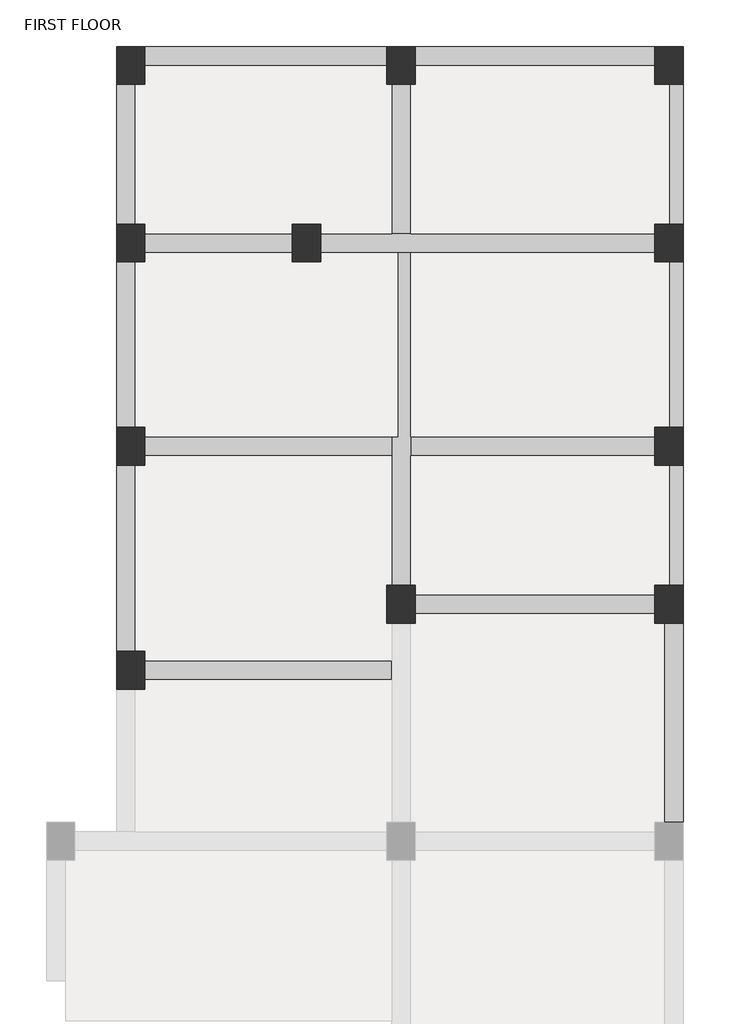
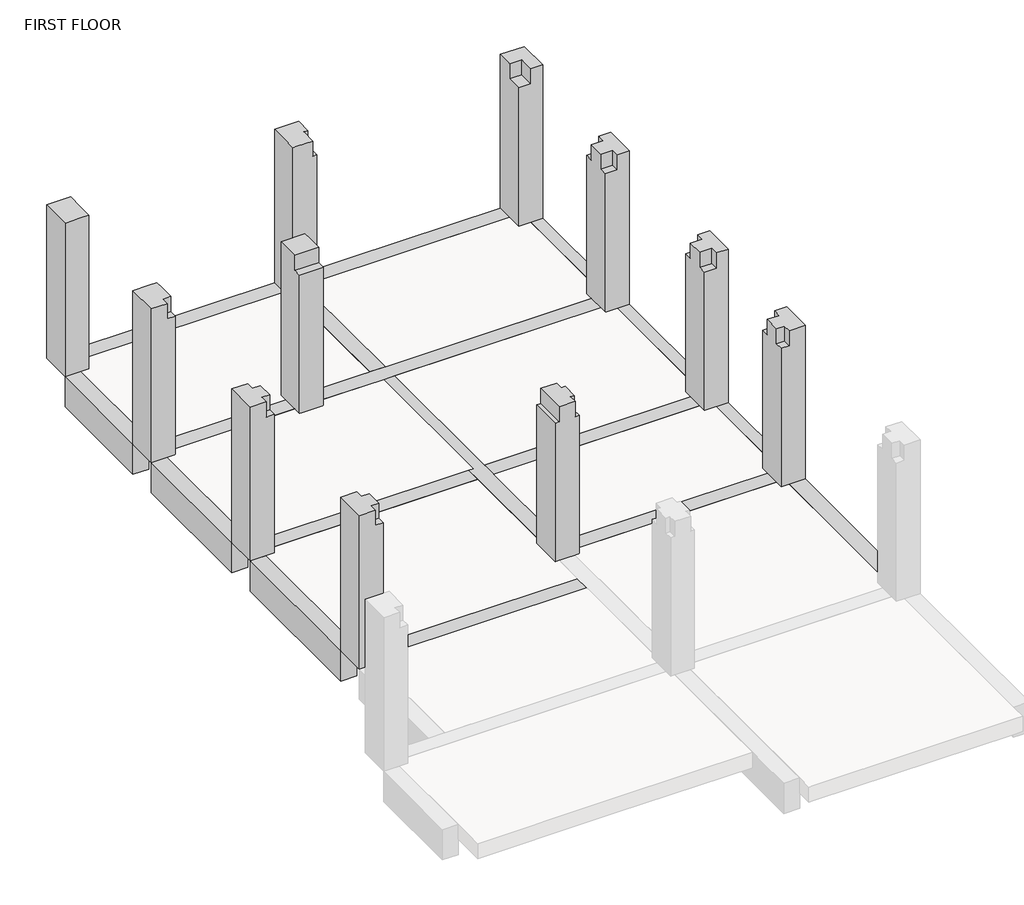
# One storey, part 2 of 2: 17 beams, 11 columns.
"""IFC4 building model written with IfcOpenShell, lengths in millimetres."""

from ifc_helpers import new_model, si_unit, frame, origin, place, context, project, spatial, polyline, outline, extrude, faceted_brep, element, save

model = new_model("IFC4")

# Units and contexts
model_context = context("Model", 3, world=origin())
ifc_project = project(units=[si_unit("LENGTHUNIT", "METRE", prefix="MILLI")], contexts=[model_context])

# Site, building, storey
site = spatial("IfcSite", under=ifc_project)
building = spatial("IfcBuilding", under=site)
storey = spatial("IfcBuildingStorey", under=building, Name="FIRST FLOOR", Elevation=3000.0)

# Beams
placement = place(None, origin())
element("IfcBeam", 1, ObjectType="M_Concrete-Rectangular Beam : 300 x 600mm", at=placement, inside=storey, context=model_context, shape_type="Brep", body=[
    faceted_brep([(-2096.635935, 10150.0657956, 3000.0), (-2096.635935, 10450.0657956, 3000.0), (-5925.9642664, 10450.0657956, 3000.0), (-5925.9642664, 10150.0657956, 3000.0), (-2096.635935, 10150.0657956, 2400.0), (-2096.635935, 10150.0657956, 2700.0), (-5925.9642664, 10150.0657956, 2700.0), (-5925.9642664, 10150.0657956, 2400.0), (-2096.635935, 10450.0657956, 2400.0), (-5925.9642664, 10450.0657956, 2400.0)], [[[0, 1, 2, 3]], [[4, 5, 0, 3, 6, 7]], [[8, 4, 7, 9]], [[1, 8, 9, 2]], [[2, 9, 7, 6, 3]], [[1, 0, 5, 4, 8]]]),
])
element("IfcBeam", 2, ObjectType="M_Concrete-Rectangular Beam : 300 x 600mm", at=placement, inside=storey, context=model_context, shape_type="SweptSolid", body=[
    extrude(outline(polyline([(2143.5134108, 10450.0657956), (2143.5134108, 10150.0657956), (-1646.635935, 10150.0657956), (-1646.635935, 10450.0657956), (2143.5134108, 10450.0657956)])), frame((0.0, 0.0, 2400.0), z_axis=(0.0, 0.0, 1.0), x_axis=(1.0, 0.0, 0.0)), (0.0, 0.0, 1.0), 600.0),
])
element("IfcBeam", 3, ObjectType="M_Concrete-Rectangular Beam : 300 x 600mm", at=placement, inside=storey, context=model_context, shape_type="Brep", body=[
    faceted_brep([(-6375.9642664, 7641.506653, 3000.0), (-6075.9642664, 7641.506653, 3000.0), (-6075.9642664, 9850.0657956, 3000.0), (-6375.9642664, 9850.0657956, 3000.0), (-6375.9642664, 7641.506653, 2400.0), (-6375.9642664, 9850.0657956, 2400.0), (-6075.9642664, 7641.506653, 2400.0), (-6075.9642664, 9850.0657956, 2400.0), (-6075.9642664, 7641.506653, 2700.0), (-6075.9642664, 9850.0657956, 2700.0)], [[[0, 1, 2, 3]], [[4, 0, 3, 5]], [[6, 4, 5, 7]], [[1, 8, 6, 7, 9, 2]], [[2, 9, 7, 5, 3]], [[1, 0, 4, 6, 8]]]),
])
element("IfcBeam", 4, ObjectType="M_Concrete-Rectangular Beam : 300 x 600mm", at=placement, inside=storey, context=model_context, shape_type="SweptSolid", body=[
    extrude(outline(polyline([(-6075.9642664, 4424.5351605), (-6375.9642664, 4424.5351605), (-6375.9642664, 7041.506653), (-6075.9642664, 7041.506653), (-6075.9642664, 4424.5351605)])), frame((0.0, 0.0, 2400.0), z_axis=(0.0, 0.0, 1.0), x_axis=(1.0, 0.0, 0.0)), (0.0, 0.0, 1.0), 600.0),
])
element("IfcBeam", 5, ObjectType="M_Concrete-Rectangular Beam : 300 x 600mm", at=placement, inside=storey, context=model_context, shape_type="SweptSolid", body=[
    extrude(outline(polyline([(-6075.9642664, 881.5941646), (-6375.9642664, 881.5941646), (-6375.9642664, 3824.5351605), (-6075.9642664, 3824.5351605), (-6075.9642664, 881.5941646)])), frame((0.0, 0.0, 2400.0), z_axis=(0.0, 0.0, 1.0), x_axis=(1.0, 0.0, 0.0)), (0.0, 0.0, 1.0), 600.0),
])
element("IfcBeam", 6, ObjectType="M_Concrete-Rectangular Beam : 300 x 600mm", at=placement, inside=storey, context=model_context, shape_type="SweptSolid", body=[
    extrude(outline(polyline([(2293.5134108, 1328.1057379), (2593.5134108, 1328.1057379), (2593.5134108, -1823.3693625), (2293.5134108, -1823.3693625), (2293.5134108, 1328.1057379)])), frame((0.0, 0.0, 2400.0), z_axis=(0.0, 0.0, 1.0), x_axis=(1.0, 0.0, 0.0)), (0.0, 0.0, 1.0), 600.0),
])
element("IfcBeam", 7, ObjectType="M_Concrete-Rectangular Beam : 300 x 600mm", at=placement, inside=storey, context=model_context, shape_type="SweptSolid", body=[
    extrude(outline(polyline([(2400.0, 2293.5134108), (2400.0, 2593.5134108), (3000.0, 2593.5134108), (3000.0, 2368.5134108), (2700.0, 2368.5134108), (2700.0, 2293.5134108), (2400.0, 2293.5134108)])), frame((0.0, 1928.1057379, 0.0), z_axis=(0.0, 1.0, 0.0), x_axis=(0.0, 0.0, 1.0)), (0.0, 0.0, 1.0), 1896.4294226),
])
element("IfcBeam", 8, ObjectType="M_Concrete-Rectangular Beam : 300 x 600mm", at=placement, inside=storey, context=model_context, shape_type="SweptSolid", body=[
    extrude(outline(polyline([(2400.0, 2293.5134108), (2400.0, 2593.5134108), (3000.0, 2593.5134108), (3000.0, 2368.5134108), (2700.0, 2368.5134108), (2700.0, 2293.5134108), (2400.0, 2293.5134108)])), frame((0.0, 4424.5351605, 0.0), z_axis=(0.0, 1.0, 0.0), x_axis=(0.0, 0.0, 1.0)), (0.0, 0.0, 1.0), 2616.9714925),
])
element("IfcBeam", 9, ObjectType="M_Concrete-Rectangular Beam : 300 x 600mm", at=placement, inside=storey, context=model_context, shape_type="SweptSolid", body=[
    extrude(outline(polyline([(2400.0, 2293.5134108), (2400.0, 2593.5134108), (3000.0, 2593.5134108), (3000.0, 2368.5134108), (2700.0, 2368.5134108), (2700.0, 2293.5134108), (2400.0, 2293.5134108)])), frame((0.0, 7641.506653, 0.0), z_axis=(0.0, 1.0, 0.0), x_axis=(0.0, 0.0, 1.0)), (0.0, 0.0, 1.0), 2208.5591426),
])
element("IfcBeam", 10, ObjectType="M_Concrete-Rectangular Beam : 300 x 600mm", at=placement, inside=storey, context=model_context, shape_type="Brep", body=[
    faceted_brep([(-3596.635935, 7191.506653, 3000.0), (-3596.635935, 7491.506653, 3000.0), (-5925.9642664, 7491.506653, 3000.0), (-5925.9642664, 7191.506653, 3000.0), (-3596.635935, 7191.506653, 2400.0), (-5925.9642664, 7191.506653, 2400.0), (-3596.635935, 7491.506653, 2400.0), (-5925.9642664, 7491.506653, 2400.0), (-3596.635935, 7491.506653, 2700.0), (-5925.9642664, 7491.506653, 2700.0)], [[[0, 1, 2, 3]], [[4, 0, 3, 5]], [[6, 4, 5, 7]], [[1, 8, 6, 7, 9, 2]], [[2, 9, 7, 5, 3]], [[1, 0, 4, 6, 8]]]),
])
element("IfcBeam", 11, ObjectType="M_Concrete-Rectangular Beam : 300 x 600mm", at=placement, inside=storey, context=model_context, shape_type="Brep", body=[
    faceted_brep([(-3146.635935, 7491.506653, 3000.0), (-3146.635935, 7191.506653, 3000.0), (-1928.7254278, 7191.506653, 3000.0), (-1721.635935, 7191.506653, 3000.0), (2143.5134108, 7191.506653, 3000.0), (2143.5134108, 7491.506653, 3000.0), (-1721.635935, 7491.506653, 3000.0), (-2021.635935, 7491.506653, 3000.0), (-3146.635935, 7491.506653, 2400.0), (-3146.635935, 7491.506653, 2700.0), (2143.5134108, 7491.506653, 2400.0), (-1721.635935, 7491.506653, 2400.0), (-2021.635935, 7491.506653, 2400.0), (-3146.635935, 7191.506653, 2400.0), (2143.5134108, 7191.506653, 2400.0), (-1721.635935, 7191.506653, 2400.0), (-2021.635935, 7191.506653, 2400.0)], [[[0, 1, 2, 3, 4, 5, 6, 7]], [[8, 9, 0, 7, 6, 5, 10, 11, 12]], [[13, 8, 12, 11, 10, 14, 15, 16]], [[1, 13, 16, 15, 14, 4, 3, 2]], [[1, 0, 9, 8, 13]], [[4, 14, 10, 5]]]),
])
element("IfcBeam", 12, ObjectType="M_Concrete-Rectangular Beam : 300 x 600mm", at=placement, inside=storey, context=model_context, shape_type="SweptSolid", body=[
    extrude(outline(polyline([(-1646.635935, 1478.1057379), (-1646.635935, 1778.1057379), (2143.5134108, 1778.1057379), (2143.5134108, 1478.1057379), (-1646.635935, 1478.1057379)])), frame((0.0, 0.0, 2400.0), z_axis=(0.0, 0.0, 1.0), x_axis=(1.0, 0.0, 0.0)), (0.0, 0.0, 1.0), 600.0),
])
element("IfcBeam", 13, ObjectType="M_Concrete-Rectangular Beam : 300 x 600mm", at=placement, inside=storey, context=model_context, shape_type="Brep", body=[
    faceted_brep([(-1721.635935, 9850.0657956, 3000.0), (-2021.635935, 9850.0657956, 3000.0), (-2021.635935, 7491.506653, 3000.0), (-1721.635935, 7491.506653, 3000.0), (-2021.635935, 9850.0657956, 2700.0), (-2021.635935, 9850.0657956, 2400.0), (-2021.635935, 7491.506653, 2400.0), (-2021.635935, 7491.506653, 2700.0), (-1721.635935, 9850.0657956, 2400.0), (-1721.635935, 7491.506653, 2400.0), (-1721.635935, 7491.506653, 2700.0)], [[[0, 1, 2, 3]], [[1, 4, 5, 6, 7, 2]], [[5, 8, 9, 6]], [[8, 0, 3, 10, 9]], [[0, 8, 5, 4, 1]], [[3, 2, 7, 6, 9, 10]]]),
])
element("IfcBeam", 14, ObjectType="M_Concrete-Rectangular Beam : 300 x 600mm", at=placement, inside=storey, context=model_context, shape_type="Brep", body=[
    faceted_brep([(-2021.635935, 1928.1057379, 3000.0), (-1721.635935, 1928.1057379, 3000.0), (-1721.635935, 3974.5351605, 3000.0), (-1721.635935, 4274.5351605, 3000.0), (-1721.635935, 7191.506653, 3000.0), (-1928.7254278, 7191.506653, 3000.0), (-1928.7254278, 4274.5351605, 3000.0), (-2021.635935, 4274.5351605, 3000.0), (-2021.635935, 3974.5351605, 3000.0), (-1721.635935, 1928.1057379, 2400.0), (-1721.635935, 3974.5351605, 2400.0), (-1721.635935, 4274.5351605, 2400.0), (-1721.635935, 7191.506653, 2400.0), (-1721.635935, 7191.506653, 2700.0), (-2021.635935, 1928.1057379, 2400.0), (-2021.635935, 3974.5351605, 2400.0), (-2021.635935, 4274.5351605, 2400.0), (-2021.635935, 7191.506653, 2400.0), (-2021.635935, 4274.5351605, 2700.0), (-2021.635935, 7191.506653, 2700.0), (-1928.7254278, 7191.506653, 2700.0), (-1928.7254278, 4274.5351605, 2700.0)], [[[0, 1, 2, 3, 4, 5, 6, 7, 8]], [[1, 9, 10, 11, 12, 13, 4, 3, 2]], [[9, 14, 15, 16, 17, 12, 11, 10]], [[14, 0, 8, 7, 18, 19, 17, 16, 15]], [[0, 14, 9, 1]], [[4, 13, 12, 17, 19, 20, 5]], [[21, 20, 19, 18]], [[20, 21, 6, 5]], [[6, 21, 18, 7]]]),
])
element("IfcBeam", 15, ObjectType="M_Concrete-Rectangular Beam : 300 x 600mm", at=placement, inside=storey, context=model_context, shape_type="Brep", body=[
    faceted_brep([(-5925.9642664, 731.5941646, 3000.0), (-5925.9642664, 431.5941646, 3000.0), (-2021.635935, 431.5941646, 3000.0), (-2021.635935, 731.5941646, 3000.0), (-5925.9642664, 431.5941646, 2400.0), (-2021.635935, 431.5941646, 2400.0), (-2021.635935, 431.5941646, 2700.0), (-5925.9642664, 731.5941646, 2400.0), (-2021.635935, 731.5941646, 2400.0), (-2021.635935, 731.5941646, 2700.0)], [[[0, 1, 2, 3]], [[1, 4, 5, 6, 2]], [[4, 7, 8, 5]], [[7, 0, 3, 9, 8]], [[0, 7, 4, 1]], [[3, 2, 6, 5, 8, 9]]]),
])
element("IfcBeam", 16, ObjectType="M_Concrete-Rectangular Beam : 300 x 600mm", at=placement, inside=storey, context=model_context, shape_type="Brep", body=[
    faceted_brep([(-5925.9642664, 4274.5351605, 3000.0), (-5925.9642664, 3974.5351605, 3000.0), (-2021.635935, 3974.5351605, 3000.0), (-2021.635935, 4274.5351605, 3000.0), (-5925.9642664, 3974.5351605, 2400.0), (-2021.635935, 3974.5351605, 2400.0), (-2021.635935, 3974.5351605, 2700.0), (-5925.9642664, 4274.5351605, 2400.0), (-2021.635935, 4274.5351605, 2400.0), (-2021.635935, 4274.5351605, 2700.0)], [[[0, 1, 2, 3]], [[1, 4, 5, 6, 2]], [[4, 7, 8, 5]], [[7, 0, 3, 9, 8]], [[0, 7, 4, 1]], [[3, 2, 6, 5, 8, 9]]]),
])
element("IfcBeam", 17, ObjectType="M_Concrete-Rectangular Beam : 300 x 600mm", at=placement, inside=storey, context=model_context, shape_type="Brep", body=[
    faceted_brep([(2143.5134108, 3974.5351605, 3000.0), (2143.5134108, 4274.5351605, 3000.0), (-1721.635935, 4274.5351605, 3000.0), (-1721.635935, 3974.5351605, 3000.0), (2143.5134108, 4274.5351605, 2400.0), (-1721.635935, 4274.5351605, 2400.0), (-1721.635935, 4274.5351605, 2700.0), (2143.5134108, 3974.5351605, 2400.0), (-1721.635935, 3974.5351605, 2400.0), (-1721.635935, 3974.5351605, 2700.0)], [[[0, 1, 2, 3]], [[1, 4, 5, 6, 2]], [[4, 7, 8, 5]], [[7, 0, 3, 9, 8]], [[0, 7, 4, 1]], [[3, 2, 6, 5, 8, 9]]]),
])

# Columns
element("IfcColumn", 18, ObjectType="M_Concrete-Rectangular-Column : 450 x 600mm", at=placement, inside=storey, context=model_context, shape_type="Brep", body=[
    faceted_brep([(-5925.9642664, 10450.0657956, 3000.0), (-5925.9642664, 9850.0657956, 3000.0), (-6375.9642664, 9850.0657956, 3000.0), (-6375.9642664, 10450.0657956, 3000.0), (-5925.9642664, 10450.0657956, 6048.0), (-5925.9642664, 10150.0657956, 6048.0), (-5925.9642664, 9850.0657956, 6048.0), (-5925.9642664, 9850.0657956, 5748.0), (-6075.9642664, 9850.0657956, 6048.0), (-6375.9642664, 9850.0657956, 6048.0), (-6375.9642664, 10450.0657956, 6048.0)], [[[0, 1, 2, 3]], [[1, 0, 4, 5, 6, 7]], [[2, 1, 7, 6, 8, 9]], [[3, 2, 9, 10]], [[0, 3, 10, 4]], [[10, 9, 8, 6, 5, 4]]]),
])
element("IfcColumn", 19, ObjectType="M_Concrete-Rectangular-Column : 450 x 600mm", at=placement, inside=storey, context=model_context, shape_type="Brep", body=[
    faceted_brep([(-5925.9642664, 7641.506653, 3000.0), (-5925.9642664, 7041.506653, 3000.0), (-6375.9642664, 7041.506653, 3000.0), (-6375.9642664, 7641.506653, 3000.0), (-5925.9642664, 7641.506653, 5748.0), (-5925.9642664, 7641.506653, 6048.0), (-5925.9642664, 7491.506653, 6048.0), (-5925.9642664, 7191.506653, 6048.0), (-5925.9642664, 7191.506653, 5748.0), (-5925.9642664, 7041.506653, 5748.0), (-6075.9642664, 7041.506653, 5748.0), (-6075.9642664, 7041.506653, 6048.0), (-6375.9642664, 7041.506653, 6048.0), (-6375.9642664, 7641.506653, 6048.0), (-6075.9642664, 7641.506653, 6048.0), (-6075.9642664, 7191.506653, 6048.0), (-6075.9642664, 7191.506653, 5748.0)], [[[0, 1, 2, 3]], [[1, 0, 4, 5, 6, 7, 8, 9]], [[2, 1, 9, 10, 11, 12]], [[3, 2, 12, 13]], [[0, 3, 13, 14, 5, 4]], [[13, 12, 11, 15, 7, 6, 5, 14]], [[16, 10, 9, 8]], [[15, 16, 8, 7]], [[16, 15, 11, 10]]]),
])
element("IfcColumn", 20, ObjectType="M_Concrete-Rectangular-Column : 450 x 600mm", at=placement, inside=storey, context=model_context, shape_type="Brep", body=[
    faceted_brep([(-5925.9642664, 4424.5351605, 3000.0), (-5925.9642664, 3824.5351605, 3000.0), (-6375.9642664, 3824.5351605, 3000.0), (-6375.9642664, 4424.5351605, 3000.0), (-5925.9642664, 4424.5351605, 5748.0), (-5925.9642664, 4274.5351605, 5748.0), (-5925.9642664, 4274.5351605, 6048.0), (-5925.9642664, 3974.5351605, 6048.0), (-5925.9642664, 3974.5351605, 5748.0), (-5925.9642664, 3824.5351605, 5748.0), (-6075.9642664, 3824.5351605, 5748.0), (-6075.9642664, 3824.5351605, 6048.0), (-6375.9642664, 3824.5351605, 6048.0), (-6375.9642664, 4424.5351605, 6048.0), (-6075.9642664, 4424.5351605, 6048.0), (-6075.9642664, 4424.5351605, 5748.0), (-6075.9642664, 3974.5351605, 6048.0), (-6075.9642664, 4274.5351605, 6048.0), (-6075.9642664, 4274.5351605, 5748.0), (-6075.9642664, 3974.5351605, 5748.0)], [[[0, 1, 2, 3]], [[1, 0, 4, 5, 6, 7, 8, 9]], [[2, 1, 9, 10, 11, 12]], [[3, 2, 12, 13]], [[0, 3, 13, 14, 15, 4]], [[13, 12, 11, 16, 7, 6, 17, 14]], [[15, 18, 5, 4]], [[18, 17, 6, 5]], [[17, 18, 15, 14]], [[19, 10, 9, 8]], [[16, 19, 8, 7]], [[19, 16, 11, 10]]]),
])
element("IfcColumn", 21, ObjectType="M_Concrete-Rectangular-Column : 450 x 600mm", at=placement, inside=storey, context=model_context, shape_type="Brep", body=[
    faceted_brep([(-5925.9642664, 881.5941646, 3000.0), (-5925.9642664, 281.5941646, 3000.0), (-6375.9642664, 281.5941646, 3000.0), (-6375.9642664, 881.5941646, 3000.0), (-5925.9642664, 881.5941646, 5748.0), (-5925.9642664, 731.5941646, 5748.0), (-5925.9642664, 731.5941646, 6048.0), (-5925.9642664, 431.5941646, 6048.0), (-5925.9642664, 431.5941646, 5748.0), (-5925.9642664, 281.5941646, 5748.0), (-6075.9642664, 281.5941646, 5748.0), (-6075.9642664, 281.5941646, 6048.0), (-6375.9642664, 281.5941646, 6048.0), (-6375.9642664, 881.5941646, 6048.0), (-6075.9642664, 881.5941646, 6048.0), (-6075.9642664, 881.5941646, 5748.0), (-6075.9642664, 431.5941646, 6048.0), (-6075.9642664, 731.5941646, 6048.0), (-6075.9642664, 731.5941646, 5748.0), (-6075.9642664, 431.5941646, 5748.0)], [[[0, 1, 2, 3]], [[1, 0, 4, 5, 6, 7, 8, 9]], [[2, 1, 9, 10, 11, 12]], [[3, 2, 12, 13]], [[0, 3, 13, 14, 15, 4]], [[13, 12, 11, 16, 7, 6, 17, 14]], [[15, 18, 5, 4]], [[18, 17, 6, 5]], [[17, 18, 15, 14]], [[19, 10, 9, 8]], [[19, 16, 11, 10]], [[16, 19, 8, 7]]]),
])
element("IfcColumn", 22, ObjectType="M_Concrete-Rectangular-Column : 450 x 600mm", at=placement, inside=storey, context=model_context, shape_type="Brep", body=[
    faceted_brep([(-3146.635935, 7641.506653, 3000.0), (-3146.635935, 7041.506653, 3000.0), (-3596.635935, 7041.506653, 3000.0), (-3596.635935, 7641.506653, 3000.0), (-3146.635935, 7641.506653, 5748.0), (-3146.635935, 7641.506653, 6048.0), (-3146.635935, 7491.506653, 6048.0), (-3146.635935, 7191.506653, 6048.0), (-3146.635935, 7191.506653, 5748.0), (-3146.635935, 7041.506653, 5748.0), (-3596.635935, 7041.506653, 5748.0), (-3596.635935, 7191.506653, 5748.0), (-3596.635935, 7191.506653, 6048.0), (-3596.635935, 7491.506653, 6048.0), (-3596.635935, 7641.506653, 6048.0), (-3596.635935, 7641.506653, 5748.0)], [[[0, 1, 2, 3]], [[1, 0, 4, 5, 6, 7, 8, 9]], [[2, 1, 9, 10]], [[3, 2, 10, 11, 12, 13, 14, 15]], [[0, 3, 15, 14, 5, 4]], [[5, 14, 13, 12, 7, 6]], [[8, 11, 10, 9]], [[11, 8, 7, 12]]]),
])
element("IfcColumn", 23, ObjectType="M_Concrete-Rectangular-Column : 450 x 600mm", at=placement, inside=storey, context=model_context, shape_type="Brep", body=[
    faceted_brep([(-1646.635935, 10450.0657956, 3000.0), (-1646.635935, 9850.0657956, 3000.0), (-2096.635935, 9850.0657956, 3000.0), (-2096.635935, 10450.0657956, 3000.0), (-1646.635935, 10450.0657956, 6048.0), (-1646.635935, 10150.0657956, 6048.0), (-1646.635935, 10150.0657956, 5748.0), (-1646.635935, 9850.0657956, 5748.0), (-1721.635935, 9850.0657956, 5748.0), (-1721.635935, 9850.0657956, 6048.0), (-2021.635935, 9850.0657956, 6048.0), (-2096.635935, 9850.0657956, 6048.0), (-2096.635935, 9850.0657956, 5748.0), (-2096.635935, 10150.0657956, 6048.0), (-2096.635935, 10450.0657956, 6048.0), (-1721.635935, 10150.0657956, 6048.0), (-1721.635935, 10150.0657956, 5748.0)], [[[0, 1, 2, 3]], [[1, 0, 4, 5, 6, 7]], [[2, 1, 7, 8, 9, 10, 11, 12]], [[3, 2, 12, 11, 13, 14]], [[0, 3, 14, 4]], [[4, 14, 13, 11, 10, 9, 15, 5]], [[16, 8, 7, 6]], [[15, 16, 6, 5]], [[16, 15, 9, 8]]]),
])
element("IfcColumn", 24, ObjectType="M_Concrete-Rectangular-Column : 450 x 600mm", at=placement, inside=storey, context=model_context, shape_type="Brep", body=[
    faceted_brep([(-1646.635935, 1928.1057379, 3000.0), (-1646.635935, 1328.1057379, 3000.0), (-2096.635935, 1328.1057379, 3000.0), (-2096.635935, 1928.1057379, 3000.0), (-1646.635935, 1928.1057379, 5748.0), (-1646.635935, 1778.1057379, 5748.0), (-1646.635935, 1778.1057379, 6048.0), (-1646.635935, 1478.1057379, 6048.0), (-1646.635935, 1478.1057379, 5748.0), (-1646.635935, 1328.1057379, 5748.0), (-1721.635935, 1328.1057379, 5748.0), (-1721.635935, 1328.1057379, 6048.0), (-2021.635935, 1328.1057379, 6048.0), (-2021.635935, 1328.1057379, 5748.0), (-2096.635935, 1328.1057379, 5748.0), (-2096.635935, 1928.1057379, 5748.0), (-2021.635935, 1928.1057379, 5748.0), (-2021.635935, 1928.1057379, 6048.0), (-1721.635935, 1928.1057379, 6048.0), (-1721.635935, 1928.1057379, 5748.0), (-1721.635935, 1778.1057379, 6048.0), (-1721.635935, 1478.1057379, 6048.0), (-1721.635935, 1778.1057379, 5748.0), (-1721.635935, 1478.1057379, 5748.0)], [[[0, 1, 2, 3]], [[1, 0, 4, 5, 6, 7, 8, 9]], [[2, 1, 9, 10, 11, 12, 13, 14]], [[3, 2, 14, 15]], [[0, 3, 15, 16, 17, 18, 19, 4]], [[6, 20, 18, 17, 12, 11, 21, 7]], [[19, 22, 5, 4]], [[22, 20, 6, 5]], [[20, 22, 19, 18]], [[23, 10, 9, 8]], [[21, 23, 8, 7]], [[23, 21, 11, 10]], [[13, 16, 15, 14]], [[16, 13, 12, 17]]]),
])
element("IfcColumn", 25, ObjectType="M_Concrete-Rectangular-Column : 450 x 600mm", at=placement, inside=storey, context=model_context, shape_type="Brep", body=[
    faceted_brep([(2593.5134108, 10450.0657956, 3000.0), (2593.5134108, 9850.0657956, 3000.0), (2143.5134108, 9850.0657956, 3000.0), (2143.5134108, 10450.0657956, 3000.0), (2593.5134108, 10450.0657956, 6048.0), (2593.5134108, 9850.0657956, 6048.0), (2368.5134108, 9850.0657956, 6048.0), (2368.5134108, 9850.0657956, 5748.0), (2143.5134108, 9850.0657956, 5748.0), (2143.5134108, 10150.0657956, 5748.0), (2143.5134108, 10150.0657956, 6048.0), (2143.5134108, 10450.0657956, 6048.0), (2368.5134108, 10150.0657956, 6048.0), (2368.5134108, 10150.0657956, 5748.0)], [[[0, 1, 2, 3]], [[1, 0, 4, 5]], [[2, 1, 5, 6, 7, 8]], [[3, 2, 8, 9, 10, 11]], [[0, 3, 11, 4]], [[5, 4, 11, 10, 12, 6]], [[7, 13, 9, 8]], [[13, 12, 10, 9]], [[12, 13, 7, 6]]]),
])
element("IfcColumn", 26, ObjectType="M_Concrete-Rectangular-Column : 450 x 600mm", at=placement, inside=storey, context=model_context, shape_type="Brep", body=[
    faceted_brep([(2593.5134108, 7641.506653, 3000.0), (2593.5134108, 7041.506653, 3000.0), (2143.5134108, 7041.506653, 3000.0), (2143.5134108, 7641.506653, 3000.0), (2593.5134108, 7641.506653, 6048.0), (2593.5134108, 7041.506653, 6048.0), (2368.5134108, 7041.506653, 6048.0), (2368.5134108, 7041.506653, 5748.0), (2143.5134108, 7041.506653, 5748.0), (2143.5134108, 7191.506653, 5748.0), (2143.5134108, 7191.506653, 6048.0), (2143.5134108, 7491.506653, 6048.0), (2143.5134108, 7491.506653, 5748.0), (2143.5134108, 7641.506653, 5748.0), (2368.5134108, 7641.506653, 5748.0), (2368.5134108, 7641.506653, 6048.0), (2368.5134108, 7491.506653, 6048.0), (2368.5134108, 7191.506653, 6048.0), (2368.5134108, 7491.506653, 5748.0), (2368.5134108, 7191.506653, 5748.0)], [[[0, 1, 2, 3]], [[1, 0, 4, 5]], [[2, 1, 5, 6, 7, 8]], [[3, 2, 8, 9, 10, 11, 12, 13]], [[0, 3, 13, 14, 15, 4]], [[5, 4, 15, 16, 11, 10, 17, 6]], [[12, 18, 14, 13]], [[18, 16, 15, 14]], [[16, 18, 12, 11]], [[7, 19, 9, 8]], [[19, 17, 10, 9]], [[17, 19, 7, 6]]]),
])
element("IfcColumn", 27, ObjectType="M_Concrete-Rectangular-Column : 450 x 600mm", at=placement, inside=storey, context=model_context, shape_type="Brep", body=[
    faceted_brep([(2593.5134108, 4424.5351605, 3000.0), (2593.5134108, 3824.5351605, 3000.0), (2143.5134108, 3824.5351605, 3000.0), (2143.5134108, 4424.5351605, 3000.0), (2593.5134108, 4424.5351605, 6048.0), (2593.5134108, 3824.5351605, 6048.0), (2368.5134108, 3824.5351605, 6048.0), (2368.5134108, 3824.5351605, 5748.0), (2143.5134108, 3824.5351605, 5748.0), (2143.5134108, 3974.5351605, 5748.0), (2143.5134108, 3974.5351605, 6048.0), (2143.5134108, 4274.5351605, 6048.0), (2143.5134108, 4274.5351605, 5748.0), (2143.5134108, 4424.5351605, 5748.0), (2368.5134108, 4424.5351605, 5748.0), (2368.5134108, 4424.5351605, 6048.0), (2368.5134108, 4274.5351605, 6048.0), (2368.5134108, 3974.5351605, 6048.0), (2368.5134108, 4274.5351605, 5748.0), (2368.5134108, 3974.5351605, 5748.0)], [[[0, 1, 2, 3]], [[1, 0, 4, 5]], [[2, 1, 5, 6, 7, 8]], [[3, 2, 8, 9, 10, 11, 12, 13]], [[0, 3, 13, 14, 15, 4]], [[5, 4, 15, 16, 11, 10, 17, 6]], [[12, 18, 14, 13]], [[18, 16, 15, 14]], [[16, 18, 12, 11]], [[7, 19, 9, 8]], [[17, 19, 7, 6]], [[19, 17, 10, 9]]]),
])
element("IfcColumn", 28, ObjectType="M_Concrete-Rectangular-Column : 450 x 600mm", at=placement, inside=storey, context=model_context, shape_type="Brep", body=[
    faceted_brep([(2593.5134108, 1928.1057379, 3000.0), (2593.5134108, 1328.1057379, 3000.0), (2143.5134108, 1328.1057379, 3000.0), (2143.5134108, 1928.1057379, 3000.0), (2593.5134108, 1928.1057379, 6048.0), (2593.5134108, 1328.1057379, 6048.0), (2293.5134108, 1328.1057379, 6048.0), (2293.5134108, 1328.1057379, 5748.0), (2143.5134108, 1328.1057379, 5748.0), (2143.5134108, 1478.1057379, 5748.0), (2143.5134108, 1478.1057379, 6048.0), (2143.5134108, 1778.1057379, 6048.0), (2143.5134108, 1778.1057379, 5748.0), (2143.5134108, 1928.1057379, 5748.0), (2368.5134108, 1928.1057379, 5748.0), (2368.5134108, 1928.1057379, 6048.0), (2368.5134108, 1778.1057379, 6048.0), (2293.5134108, 1478.1057379, 6048.0), (2368.5134108, 1778.1057379, 5748.0), (2293.5134108, 1478.1057379, 5748.0)], [[[0, 1, 2, 3]], [[1, 0, 4, 5]], [[2, 1, 5, 6, 7, 8]], [[3, 2, 8, 9, 10, 11, 12, 13]], [[0, 3, 13, 14, 15, 4]], [[5, 4, 15, 16, 11, 10, 17, 6]], [[12, 18, 14, 13]], [[18, 16, 15, 14]], [[16, 18, 12, 11]], [[7, 19, 9, 8]], [[19, 17, 10, 9]], [[17, 19, 7, 6]]]),
])

save(model, "model.ifc")

# Revit data of these elements
# Type "M_Concrete-Rectangular Beam : 300 x 600mm"
#   Length [instance default] = 1524 mm
#   b = 300 mm
#   h = 600 mm
#   Structural Material [instance default] = Concrete, Cast-in-Place gray
#   Assembly Code = ""
# Type "M_Concrete-Rectangular-Column : 450 x 600mm"
#   b = 450 mm
#   h = 600 mm
#   Structural Material [instance default] = Concrete, Cast-in-Place gray
# Elements 1, 2, 3, 4, 5, 6, 7, 8, 9, 10, 11, 12, 13, 14, 15, 16, 17 (IfcBeam, "M_Concrete-Rectangular Beam : 300 x 600mm")
#   Structural Material = Concrete, Cast-in-Place gray
#   Phase Created = New Construction
#   Materials on its faces: "Concrete, Cast-in-Place gray"
# Elements 18, 19, 20, 21, 22, 23, 24, 25, 26, 27, 28 (IfcColumn, "M_Concrete-Rectangular-Column : 450 x 600mm")
#   Structural Material = Concrete, Cast-in-Place gray
#   Phase Created = New Construction
#   Materials on its faces: "Concrete, Cast-in-Place gray"
# Materials
#   "Concrete, Cast-in-Place gray": class "Concrete", colour RGB 192 192 192, transparency 0, Description = "Cast-in-place concrete", Cost = 0
